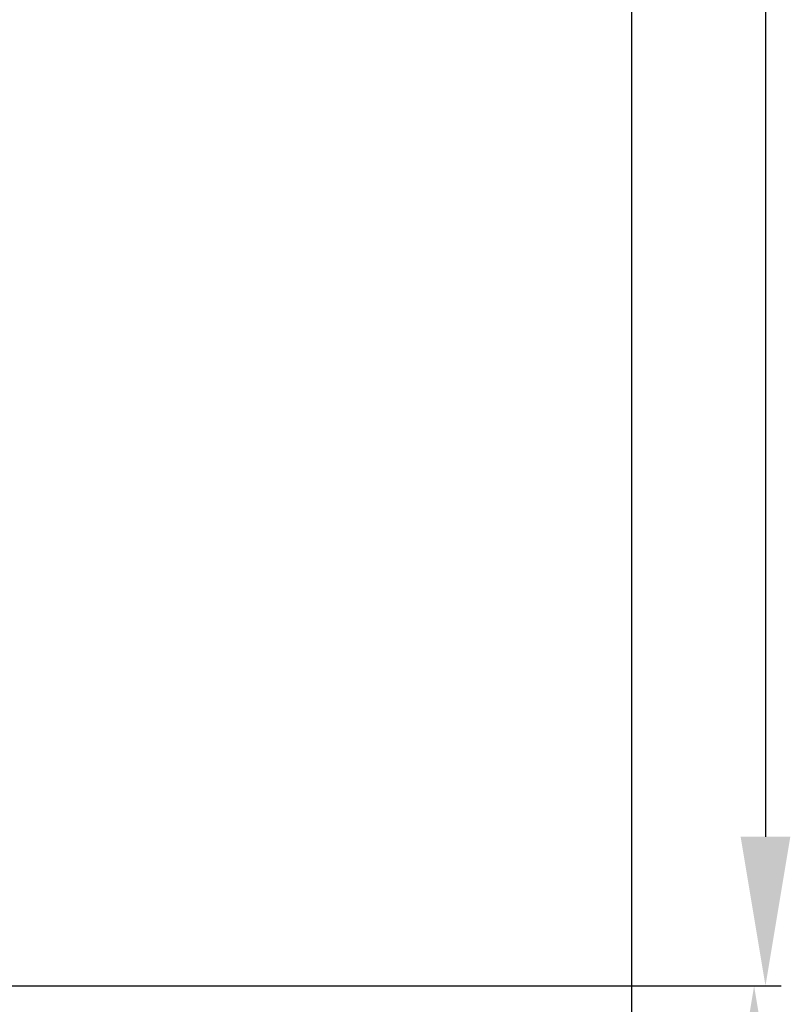
# Model space of a CAD drawing. Units: inches. Extents: x 2083 to 3317, y 1141 to 2115.
# Tile 251 of 256: x 3130 to 3192, y 1485 to 1564. Entities that reach past the tile are written whole.
import ezdxf

# ---------------------------------------------------------------- set-up
doc = ezdxf.new("R2010")
doc.units = ezdxf.units.IN
doc.layers.add('A-ANNO-DIMS', color=2, linetype='Continuous', lineweight=18)
doc.styles.get("Standard").update_dxf_attribs({"font": 'arial.ttf'})
doc.dimstyles.new('ISO-25', dxfattribs={"dimtxt": 12, "dimasz": 12, "dimexe": 1.25, "dimexo": 0.625, "dimtad": 1, "dimlunit": 3, "dimtxsty": 'Standard', "dimcen": 2.5, "dimadec": 0, "dimazin": 0, "dimtfac": 1, "dimtmove": 0, "dimatfit": 3, "dimfxl": 1, "dimarcsym": 0})

# ---------------------------------------------------------------- blocks, each defined once
blk = doc.blocks.new('*D8')
at = {"layer": 'A-ANNO-DIMS', "color": 0, "lineweight": -2, "transparency": 16777216}
for p, q in [((3127.585, 1702.761), (3191.318, 1702.761)), ((3190.068, 1690.761), (3190.068, 1498.761)), ((3127.585, 1486.761), (3191.318, 1486.761))]:
    blk.add_line(p, q, dxfattribs=at)
at = {"layer": 'A-ANNO-DIMS', "color": 0, "transparency": 16777216}
for points in [[(3188.068, 1690.761), (3192.068, 1690.761), (3190.068, 1702.761)], [(3188.068, 1498.761), (3192.068, 1498.761), (3190.068, 1486.761)]]:
    blk.add_solid(points, dxfattribs=at)
at = {"layer": 'Defpoints', "color": 0, "transparency": 16777216}
for p in [(3126.96, 1702.761), (3126.96, 1486.761), (3190.068, 1486.761)]:
    blk.add_point(p, dxfattribs=at)
at = {"layer": 'A-ANNO-DIMS', "color": 0, "transparency": 16777216, "insert": (3183.316, 1594.761), "char_height": 12, "attachment_point": 5, "rotation": 90}
blk.add_mtext("18'", dxfattribs=at)
blk = doc.blocks.new('*D9')
at = {"layer": 'A-ANNO-DIMS', "color": 0, "lineweight": -2, "transparency": 16777216}
for p, q in [((3127.585, 1486.761), (3190.403, 1486.761)), ((3189.153, 1474.761), (3189.153, 1275.261)), ((3127.585, 1263.261), (3190.403, 1263.261))]:
    blk.add_line(p, q, dxfattribs=at)
at = {"layer": 'A-ANNO-DIMS', "color": 0, "transparency": 16777216}
for points in [[(3187.153, 1474.761), (3191.153, 1474.761), (3189.153, 1486.761)], [(3187.153, 1275.261), (3191.153, 1275.261), (3189.153, 1263.261)]]:
    blk.add_solid(points, dxfattribs=at)
at = {"layer": 'Defpoints', "color": 0, "transparency": 16777216}
for p in [(3126.96, 1486.761), (3126.96, 1263.261), (3189.153, 1263.261)]:
    blk.add_point(p, dxfattribs=at)
at = {"layer": 'A-ANNO-DIMS', "color": 0, "transparency": 16777216, "insert": (3182.401, 1375.011), "char_height": 12, "attachment_point": 5, "rotation": 90}
blk.add_mtext('18\'-7.5"', dxfattribs=at)
blk = doc.blocks.new('*D35')
at = {"layer": 'A-ANNO-DIMS', "color": 0, "lineweight": -2, "transparency": 16777216}
for p, q in [((3127.585, 2020.761), (3180.56, 2020.761)), ((3179.31, 1275.261), (3179.31, 2008.761)), ((3127.585, 1263.261), (3180.56, 1263.261))]:
    blk.add_line(p, q, dxfattribs=at)
at = {"layer": 'A-ANNO-DIMS', "color": 0, "transparency": 16777216}
for points in [[(3177.31, 2008.761), (3181.31, 2008.761), (3179.31, 2020.761)], [(3177.31, 1275.261), (3181.31, 1275.261), (3179.31, 1263.261)]]:
    blk.add_solid(points, dxfattribs=at)
at = {"layer": 'Defpoints', "color": 0, "transparency": 16777216}
for p in [(3126.96, 2020.761), (3179.31, 2020.761), (3126.96, 1263.261)]:
    blk.add_point(p, dxfattribs=at)
at = {"layer": 'A-ANNO-DIMS', "color": 0, "transparency": 16777216, "insert": (3172.476, 1642.011), "char_height": 12, "attachment_point": 5, "rotation": 90}
blk.add_mtext('63\'-1 1/2"', dxfattribs=at)

msp = doc.modelspace()

# ---------------------------------------------------------------- dimensions: what is measured, and where the dimension line sits
at = {"layer": 'A-ANNO-DIMS'}
for base, p1, p2, override, picture, middle in [((3179.31, 2020.761), (3126.96, 1263.261), (3126.96, 2020.761), {"dimdec": 1, "dimlfac": 1, "dimrnd": 0, "dimzin": 1, "dimdsep": 46, "dimlunit": 4, "dimfrac": 2}, '*D35', (3172.476, 1642.011)), ((3190.068, 1486.761), (3126.96, 1702.761), (3126.96, 1486.761), {"dimclrd": 0, "dimclre": 0, "dimclrt": 0}, '*D8', (3183.316, 1594.761)), ((3189.153, 1263.261), (3126.96, 1486.761), (3126.96, 1263.261), {"dimclrd": 0, "dimclre": 0, "dimclrt": 0}, '*D9', (3182.401, 1375.011))]:
    dim = msp.add_linear_dim(base=base, p1=p1, p2=p2, angle=90, dimstyle='ISO-25', override=override, dxfattribs=at)
    dim.commit()
    dim.dimension.update_dxf_attribs({"geometry": picture, "text_midpoint": middle})

doc.saveas('drawing.dxf')
